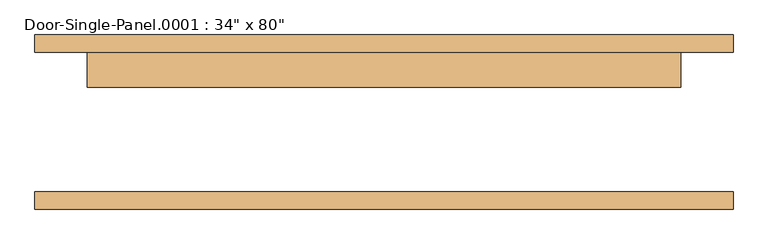
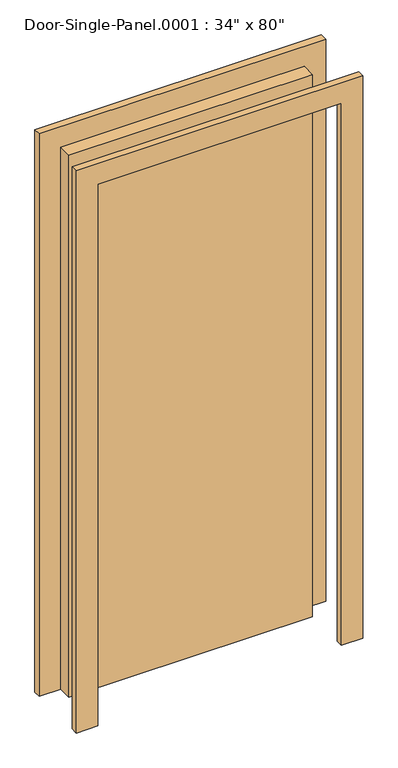
"""IFC4 building model written with IfcOpenShell, lengths in millimetres: door geometry."""

from ifc_helpers import new_model, si_unit, frame, origin, origin_with_axes, place, context, project, spatial, polyline, outline, extrude, source, transform, mapped, element, save


def door_10fd3a06(model_context):
    return source(origin(), model_context, "Body", "SweptSolid", [
        extrude(outline(polyline([(431.8, 50.8), (-431.8, 50.8), (-431.8, 101.6), (431.8, 101.6), (431.8, 50.8)])), origin_with_axes(), (0.0, 0.0, 1.0), 2032.0),
        extrude(outline(polyline([(2108.2, -508.0), (0.0, -508.0), (0.0, -431.8), (2032.0, -431.8), (2032.0, 431.8), (0.0, 431.8), (0.0, 508.0), (2108.2, 508.0), (2108.2, -508.0)])), frame((0.0, 101.6, 0.0), z_axis=(0.0, 1.0, 0.0), x_axis=(0.0, 0.0, 1.0)), (0.0, 0.0, 1.0), 25.4),
        extrude(outline(polyline([(2108.2, 508.0), (2108.2, -508.0), (0.0, -508.0), (0.0, -431.8), (2032.0, -431.8), (2032.0, 431.8), (0.0, 431.8), (0.0, 508.0), (2108.2, 508.0)])), frame((0.0, -127.0, 0.0), z_axis=(0.0, 1.0, 0.0), x_axis=(0.0, 0.0, 1.0)), (0.0, 0.0, 1.0), 25.4),
    ])


if __name__ == "__main__":
    model = new_model("IFC4")
    model_context = context("Model", 3, world=origin())
    ifc_project = project(units=[si_unit("LENGTHUNIT", "METRE", prefix="MILLI")], contexts=[model_context])
    site = spatial("IfcSite", under=ifc_project)
    building = spatial("IfcBuilding", under=site)
    placement = place(None, origin())
    door_shape = door_10fd3a06(model_context)
    element("IfcDoor", 1, ObjectType="Door-Single-Panel.0001 : 34\" x 80\"", at=placement, inside=building, context=model_context, shape_type="MappedRepresentation", body=[
        mapped(door_shape, transform((0.0, 0.0, 0.0), x_axis=(1.0, 0.0, 0.0), y_axis=(0.0, 1.0, 0.0), z_axis=(0.0, 0.0, 1.0))),
    ])
    save(model, "model.ifc")

# Revit data of these elements
# Type "Door-Single-Panel.0001 : 34\" x 80\""
#   Type Mark = "9"
#   Construction Type Id = "DOOR"
#   Assembly Code = "C1020300"
#   Analytic Construction = "Wooden"
#   Thickness = 0' - 2"
#   Thermal Resistance (R) = 0.455703 (m²·K)/W
#   Swing Angle [instance default] = 90.00°
#   Heat Transfer Coefficient (U) = 2.19465 W/(m²·K)
#   Height = 6' - 8"
#   Trim Projection Ext = 0' - 1"
#   Trim Projection Int = 0' - 1"
#   Trim Width = 0' - 3"
#   Width = 2' - 10"
#   Panel Material = Wood - Birch - Solid Stained Light Low Gloss
#   Trim Material = Paint - Sienna
#   Visual Light Transmittance = 0
#   Solar Heat Gain Coefficient = 0
#   Function = (empty or 0)
#   Wall Closure = (empty or 0)
# Element 1 (IfcDoor, "Door-Single-Panel.0001 : 34\" x 80\"")
#   Materials on its faces: "Paint - Sienna", "Wood - Birch - Solid Stained Light Low Gloss"
# Materials
#   "Wood - Birch - Solid Stained Light Low Gloss": class "Wood", colour RGB 210 159 95, transparency 0, Cost = 0
#   "Paint - Sienna": colour RGB 118 70 51, transparency 0, Cost = 0
